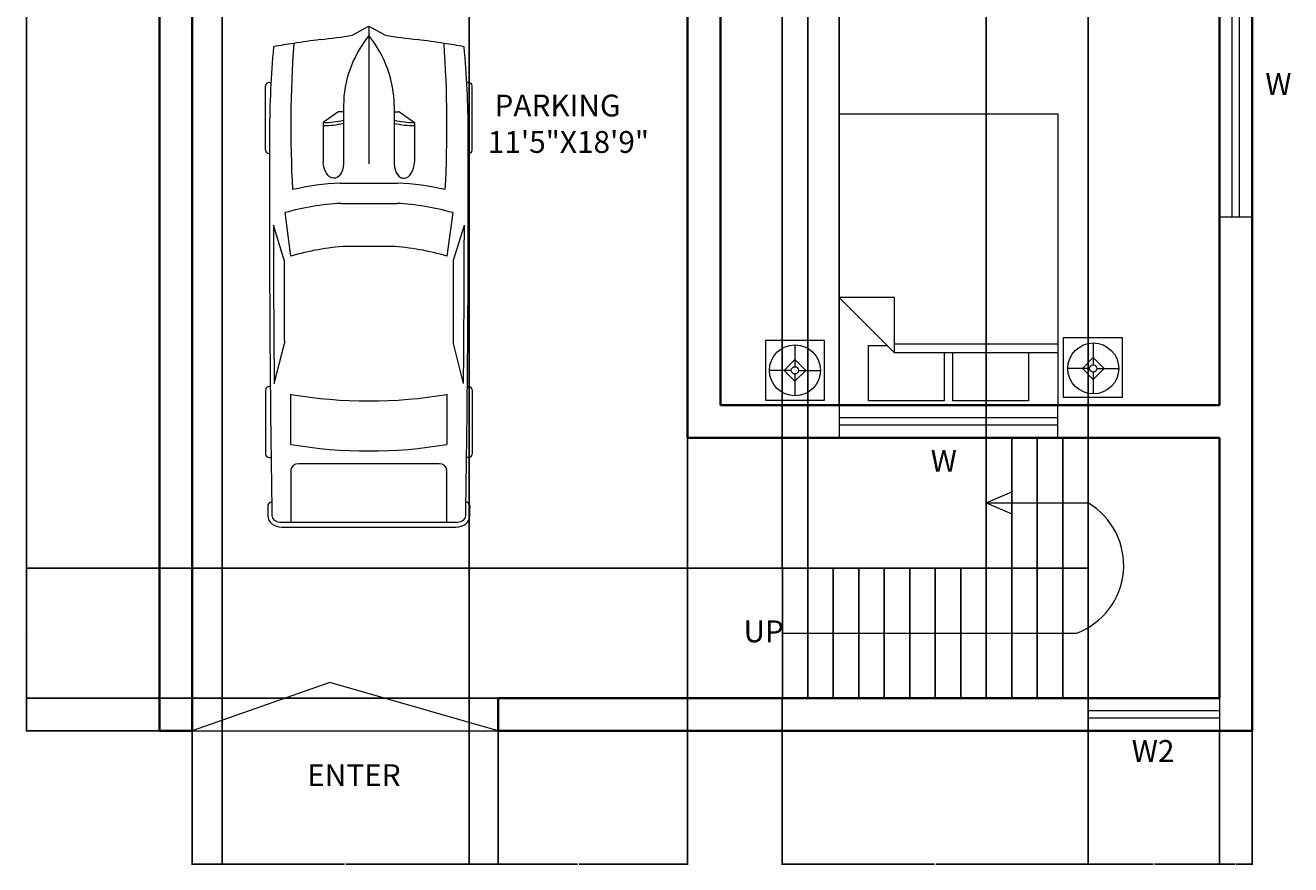
# Model space of a CAD drawing. Units: inches. Extents: x 2523 to 5630, y 2079 to 4208.
# Tile 1 of 3: x 2523 to 2870, y 2079 to 2309. Entities that reach past the tile are written whole.
import ezdxf

# ---------------------------------------------------------------- set-up
doc = ezdxf.new("R2010")
doc.units = ezdxf.units.IN
for name, color, linetype, lineweight in [('A-ANNO-DIMS', 2, 'Continuous', 18), ('A-ANNO-SYMB', 2, 'Continuous', 18), ('A-ANNO-TEXT', 7, 'Continuous', 18), ('A-AREA-IDEN', 7, 'Continuous', 25), ('A-EQPM-VEHC', 9, 'Continuous', 13), ('A-FLOR-STRS', 7, 'Continuous', 25), ('A-FURN', 8, 'Continuous', 18), ('A-GLAZ', 4, 'Continuous', 18), ('A-WALL', 7, 'Continuous', 35)]:
    doc.layers.add(name, color=color, linetype=linetype, lineweight=lineweight)
doc.styles.get("Standard").update_dxf_attribs({"font": 'arial.ttf'})
doc.dimstyles.get("Standard").update_dxf_attribs({"dimtxt": 0.18, "dimasz": 0.18, "dimexe": 0.18, "dimexo": 0.0625, "dimgap": 0.09, "dimtad": 0, "dimtih": 1, "dimtoh": 1, "dimdec": 4, "dimzin": 0, "dimdsep": 46, "dimtxsty": 'Standard', "dimcen": 0.09, "dimadec": 0, "dimazin": 0, "dimtfac": 1, "dimtdec": 4, "dimtofl": 0, "dimtmove": 0, "dimatfit": 3, "dimfxl": 1, "dimtolj": 1, "dimtzin": 0, "dimarcsym": 0})

# ---------------------------------------------------------------- blocks, each defined once
blk = doc.blocks.new('Bed - Queen')
for p, q in [((0, -80.00003), (0, 0)), ((0, 0), (59.99999, 0)), ((59.99999, 0), (59.99999, -80.00003)), ((7.99999, -1.2), (28.79998, -1.2)), ((7.99999, -14.4), (7.99999, -1.2)), ((28.79998, -1.2), (28.79998, -14.4)), ((31.19999, -1.2), (51.99999, -1.2)), ((31.19999, -14.4), (31.19999, -1.2)), ((51.99999, -1.2), (51.99999, -16.4)), ((0, -14.4), (44.8, -14.4)), ((44.8, -16.8), (0, -16.8)), ((59.99999, -29.6), (44.8, -14.4)), ((44.8, -14.4), (44.8, -29.6)), ((51.99999, -16.4), (46.79936, -16.4)), ((44.8, -29.6), (59.99999, -29.6)), ((59.99999, -80.00003), (0, -80.00003))]:
    blk.add_line(p, q)
blk = doc.blocks.new('Lamp - Table')
for p, q in [((0, 7), (0, 1)), ((-1, 0), (-7, 0)), ((0, 3), (-3, 0)), ((-3, 0), (0, -3)), ((3, 0), (0, 3)), ((0, -3), (3, 0)), ((1, 0), (7, 0)), ((0, -1), (0, -7))]:
    blk.add_line(p, q)
for radius in [7, 1]:
    blk.add_circle((0, 0), radius)
blk = doc.blocks.new('*U9')
for p, q in [((46.55, 38.89), (22.35, 38.89)), ((136.7, 38.89), (160.9, 38.89)), ((21.1, 37.41), (21.1, 36.83)), ((47.8, 37.39), (47.8, 37.41)), ((87.99, 31.87), (74.76, 35.92)), ((134.31, 35.6), (119.29, 31.78)), ((135.45, 37.07), (135.45, 37.41)), ((162.15, 37.41), (162.15, 36.77)), ((186.47, -33.5), (186.47, 33.5)), ((70.03, 31.54), (86.41, 29.35)), ((138.42, 29.35), (157.25, 29.35)), ((186.47, 29.35), (167.01, 29.35)), ((188.4, -32.76), (188.4, 32.76)), ((164.52, 26.39), (164.52, -26.39)), ((32.27, 11.63), (36.13, 17.17)), ((36.13, 17.17), (50.94, 17.17)), ((32.12, 9.51), (32.12, 11.15)), ((58.92, -10.77), (58.92, 10.77)), ((66.55, -10.53), (66.55, 10.53)), ((186.47, -10.53), (186.47, 10.53)), ((3.27, 6.13), (0.1, 0.41)), ((29.77, 9.51), (51.68, 9.51)), ((82.74, 8.5), (82.74, -8.5)), ((0, 0), (51.68, 0)), ((0.1, -0.41), (3.27, -6.13)), ((29.77, -9.51), (51.68, -9.51)), ((32.12, -9.51), (32.12, -11.15)), ((32.27, -11.63), (36.13, -17.17)), ((36.13, -17.17), (50.94, -17.17)), ((86.41, -29.35), (70.03, -31.54)), ((87.99, -31.87), (74.76, -35.92)), ((134.31, -35.6), (119.29, -31.78)), ((157.25, -29.35), (138.42, -29.35)), ((167.01, -29.35), (186.47, -29.35)), ((21.1, -37.41), (21.1, -36.83)), ((47.8, -37.39), (47.8, -37.41)), ((135.45, -37.07), (135.45, -37.41)), ((162.15, -37.41), (162.15, -36.77)), ((46.55, -38.89), (22.35, -38.89)), ((136.7, -38.89), (160.9, -38.89))]:
    blk.add_line(p, q)
for centre, major_axis, ratio, start_param, end_param in [((22.35, 37.41), (0, -1.48), 0.842304, 3.141593, 4.712389), ((46.55, 37.41), (0, 1.48), 0.842304, -1.570796, 0), ((136.7, 37.41), (0, -1.48), 0.842304, 3.141593, 4.712389), ((160.9, 37.41), (0, 1.48), 0.842304, -1.570796, 0), ((266.03, -27.52), (0, 313.31), 0.842304, 1.367076, 1.39176), ((41.19, -490.86), (0, 528.23), 0.842304, 0.00281, 0.075598), ((64.48, -10555.62), (0, 10593.03), 0.842304, -0.013397, 0.002797), ((64.48, -10555.62), (0, -10591.55), 0.842304, 3.133765, 3.140441), ((180.63, 35.84), (0, 2.22), 0.842304, -0.013017, 1.249894), ((64.48, -10556.36), (0, 10595.31), 0.842304, -0.013397, -0.013017), ((183.98, 33.5), (0, -2.96), 0.842304, 1.570796, 3.128196), ((183.98, 32.76), (0, -5.25), 0.842304, 1.570796, 3.128196), ((37.47, -593.96), (0, -623.33), 0.842304, 3.096046, 3.200911), ((134.4, 5.39), (0, -89.78), 0.842304, 4.449482, 4.652344), ((135.29, 5.39), (0, 81.77), 0.842304, 1.245306, 1.50788), ((149.6, 2.8), (0, -79.58), 0.842304, 4.372215, 4.640744), ((95.79, -3666.35), (0, -3698.24), 0.842304, 3.134049, 3.144098), ((17.08, 0), (0, 147.02), 0.842304, 4.511394, 4.913384), ((35.91, 0), (0, 147.02), 0.842304, 4.511394, 4.913384), ((167.01, 26.39), (0, 2.96), 0.842304, 0, 1.570796), ((259.18, -27.52), (0, -305.3), 0.842304, 4.528606, 4.561838), ((-204.49, 52.4), (0, -250.96), 0.842304, 1.385369, 1.434372), ((13.04, 17.01), (0, 27.42), 0.842304, 4.435146, 4.718221), ((14.2, 17.01), (0, 27.42), 0.842304, 4.435146, 4.718221), ((50.79, 13.34), (6.34, -0.36), 0.603834, -1.395552, 1.581315), ((32.75, 11.15), (0, 0.74), 0.842304, 0.879714, 1.570796), ((29.77, -46.66), (0, 56.17), 0.842304, 0, 0.590319), ((0.62, 0), (0, -0.74), 0.842304, 4.131459, 5.293319), ((29.77, 46.66), (0, 56.17), 0.842304, 2.551274, 3.141593), ((-204.49, -52.4), (0, 250.96), 0.842304, -1.434372, -1.385369), ((13.04, -17.01), (0, -27.42), 0.842304, 1.564964, 1.848039), ((14.2, -17.01), (0, -27.42), 0.842304, 1.564964, 1.848039), ((149.6, -2.8), (0, -79.58), 0.842304, -1.499151, -1.230623), ((32.75, -11.15), (0, -0.74), 0.842304, 4.712389, 5.403472), ((134.4, -5.39), (0, -89.78), 0.842304, -1.510751, -1.307889), ((135.29, -5.39), (0, -81.77), 0.842304, -1.50788, -1.245306), ((259.18, 27.52), (0, 305.3), 0.842304, 1.721348, 1.754579), ((266.03, 27.52), (0, 313.31), 0.842304, 1.749832, 1.774517), ((37.47, 593.96), (0, -623.33), 0.842304, -0.059319, 0.045547), ((167.01, -26.39), (0, -2.96), 0.842304, 4.712389, 6.283185), ((95.79, 3666.35), (0, -3698.24), 0.842304, -0.002505, 0.007544), ((183.98, -32.76), (0, -5.25), 0.842304, 0.013397, 1.570796), ((41.19, 490.86), (0, -528.23), 0.842304, -0.075598, -0.00281), ((22.35, -37.41), (0, 1.48), 0.842304, 1.570796, 3.141593), ((64.48, 10555.62), (0, 10593.03), 0.842304, 3.138796, 3.15499), ((46.55, -37.41), (0, -1.48), 0.842304, 0, 1.570796), ((64.48, 10555.62), (0, -10591.55), 0.842304, 0.001152, 0.007828), ((136.7, -37.41), (0, -1.48), 0.842304, -1.570796, 0), ((160.9, -37.41), (0, 1.48), 0.842304, 3.141593, 4.712389), ((180.63, -35.84), (0, -2.22), 0.842304, -1.249894, 0.013017), ((64.48, 10556.36), (0, 10595.31), 0.842304, 3.15461, 3.15499), ((183.98, -33.5), (0, 2.96), 0.842304, 3.15499, 4.712389)]:
    blk.add_ellipse(centre, major_axis=major_axis, ratio=ratio, start_param=start_param, end_param=end_param)
at = {"extrusion": (0, 0, -1)}
blk.add_ellipse((50.79, -13.34), major_axis=(6.34, 0.36), ratio=0.603834, start_param=-1.395552, end_param=1.581315, dxfattribs=at)
blk = doc.blocks.new('WIN-W-60IN')
for p, q in [((60, 5.5), (0, 5.5)), ((60, 3.5), (0, 3.5))]:
    blk.add_line(p, q)
blk.add_lwpolyline([(0, 0), (60, 0), (60, 9), (0, 9)], close=True)
blk = doc.blocks.new('TABLE-BEDSIDE')
blk.add_lwpolyline([(0, 0), (16.27, 0), (16.27, 16.36), (0, 16.36)], close=True)
blk = doc.blocks.new('*D33')
at = {"layer": 'A-ANNO-DIMS', "color": 0, "lineweight": -2, "transparency": 16777216}
for p, q in [((2559.63, 2775.33), (2522.96, 2775.33)), ((2523.14, 2775.15), (2523.14, 2445.52)), ((2523.14, 2115.51), (2523.14, 2445.15)), ((2559.63, 2115.33), (2522.96, 2115.33))]:
    blk.add_line(p, q, dxfattribs=at)
at = {"layer": 'A-ANNO-DIMS', "color": 0, "transparency": 16777216}
for points in [[(2523.11, 2775.15), (2523.17, 2775.15), (2523.14, 2775.33)], [(2523.11, 2115.51), (2523.17, 2115.51), (2523.14, 2115.33)]]:
    blk.add_solid(points, dxfattribs=at)
at = {"layer": 'Defpoints', "color": 0, "transparency": 16777216}
for p in [(2523.14, 2775.33), (2559.69, 2775.33), (2559.69, 2115.33)]:
    blk.add_point(p, dxfattribs=at)
at = {"layer": 'A-ANNO-DIMS', "color": 0, "transparency": 16777216, "insert": (2523.14, 2445.33), "char_height": 0.18, "attachment_point": 5}
blk.add_mtext('\\A1;660', dxfattribs=at)
blk = doc.blocks.new('*D34')
at = {"layer": 'A-ANNO-DIMS', "color": 0, "lineweight": -2, "transparency": 16777216}
for p, q in [((2568.69, 2115.27), (2568.69, 2078.6)), ((2652.69, 2115.27), (2652.69, 2078.6)), ((2568.87, 2078.78), (2610.47, 2078.78)), ((2652.51, 2078.78), (2610.91, 2078.78))]:
    blk.add_line(p, q, dxfattribs=at)
at = {"layer": 'A-ANNO-DIMS', "color": 0, "transparency": 16777216}
for points in [[(2568.87, 2078.81), (2568.87, 2078.75), (2568.69, 2078.78)], [(2652.51, 2078.81), (2652.51, 2078.75), (2652.69, 2078.78)]]:
    blk.add_solid(points, dxfattribs=at)
at = {"layer": 'Defpoints', "color": 0, "transparency": 16777216}
for p in [(2568.69, 2115.33), (2652.69, 2115.33), (2652.69, 2078.78)]:
    blk.add_point(p, dxfattribs=at)
at = {"layer": 'A-ANNO-DIMS', "color": 0, "transparency": 16777216, "insert": (2610.69, 2078.78), "char_height": 0.18, "attachment_point": 5}
blk.add_mtext('\\A1;84', dxfattribs=at)
blk = doc.blocks.new('*D35')
at = {"layer": 'A-ANNO-DIMS', "color": 0, "lineweight": -2, "transparency": 16777216}
for p, q in [((2814.69, 2115.27), (2814.69, 2078.6)), ((2850.69, 2115.27), (2850.69, 2078.6)), ((2814.87, 2078.78), (2832.47, 2078.78)), ((2850.51, 2078.78), (2832.91, 2078.78))]:
    blk.add_line(p, q, dxfattribs=at)
at = {"layer": 'A-ANNO-DIMS', "color": 0, "transparency": 16777216}
for points in [[(2814.87, 2078.81), (2814.87, 2078.75), (2814.69, 2078.78)], [(2850.51, 2078.81), (2850.51, 2078.75), (2850.69, 2078.78)]]:
    blk.add_solid(points, dxfattribs=at)
at = {"layer": 'Defpoints', "color": 0, "transparency": 16777216}
for p in [(2814.69, 2115.33), (2850.69, 2115.33), (2850.69, 2078.78)]:
    blk.add_point(p, dxfattribs=at)
at = {"layer": 'A-ANNO-DIMS', "color": 0, "transparency": 16777216, "insert": (2832.69, 2078.78), "char_height": 0.18, "attachment_point": 5}
blk.add_mtext('\\A1;36', dxfattribs=at)
blk = doc.blocks.new('*D36')
at = {"layer": 'A-ANNO-DIMS', "color": 0, "lineweight": -2, "transparency": 16777216}
for p, q in [((2704.69, 2353.27), (2704.69, 2078.6)), ((2644.69, 2348.77), (2644.69, 2078.6)), ((2644.87, 2078.78), (2674.47, 2078.78)), ((2704.51, 2078.78), (2674.91, 2078.78))]:
    blk.add_line(p, q, dxfattribs=at)
at = {"layer": 'A-ANNO-DIMS', "color": 0, "transparency": 16777216}
for points in [[(2644.87, 2078.81), (2644.87, 2078.75), (2644.69, 2078.78)], [(2704.51, 2078.81), (2704.51, 2078.75), (2704.69, 2078.78)]]:
    blk.add_solid(points, dxfattribs=at)
at = {"layer": 'Defpoints', "color": 0, "transparency": 16777216}
for p in [(2704.69, 2353.33), (2644.69, 2348.83), (2704.69, 2078.78)]:
    blk.add_point(p, dxfattribs=at)
at = {"layer": 'A-ANNO-DIMS', "color": 0, "transparency": 16777216, "insert": (2674.69, 2078.78), "char_height": 0.18, "attachment_point": 5}
blk.add_mtext('\\A1;60', dxfattribs=at)
blk = doc.blocks.new('*D37')
at = {"layer": 'A-ANNO-DIMS', "color": 0, "lineweight": -2, "transparency": 16777216}
for p, q in [((2850.69, 2115.27), (2850.69, 2078.6)), ((2859.69, 2115.27), (2859.69, 2078.6)), ((2850.87, 2078.78), (2855.04, 2078.78)), ((2859.51, 2078.78), (2855.34, 2078.78))]:
    blk.add_line(p, q, dxfattribs=at)
at = {"layer": 'A-ANNO-DIMS', "color": 0, "transparency": 16777216}
for points in [[(2850.87, 2078.81), (2850.87, 2078.75), (2850.69, 2078.78)], [(2859.51, 2078.81), (2859.51, 2078.75), (2859.69, 2078.78)]]:
    blk.add_solid(points, dxfattribs=at)
at = {"layer": 'Defpoints', "color": 0, "transparency": 16777216}
for p in [(2850.69, 2115.33), (2859.69, 2115.33), (2859.69, 2078.78)]:
    blk.add_point(p, dxfattribs=at)
at = {"layer": 'A-ANNO-DIMS', "color": 0, "transparency": 16777216, "insert": (2855.19, 2078.78), "char_height": 0.18, "attachment_point": 5}
blk.add_mtext('\\A1;9', dxfattribs=at)
blk = doc.blocks.new('*D38')
at = {"layer": 'A-ANNO-DIMS', "color": 0, "lineweight": -2, "transparency": 16777216}
for p, q in [((2730.69, 2124.27), (2730.69, 2078.6)), ((2814.69, 2124.27), (2814.69, 2078.6)), ((2730.87, 2078.78), (2772.47, 2078.78)), ((2814.51, 2078.78), (2772.91, 2078.78))]:
    blk.add_line(p, q, dxfattribs=at)
at = {"layer": 'A-ANNO-DIMS', "color": 0, "transparency": 16777216}
for points in [[(2730.87, 2078.81), (2730.87, 2078.75), (2730.69, 2078.78)], [(2814.51, 2078.81), (2814.51, 2078.75), (2814.69, 2078.78)]]:
    blk.add_solid(points, dxfattribs=at)
at = {"layer": 'Defpoints', "color": 0, "transparency": 16777216}
for p in [(2730.69, 2124.33), (2814.69, 2124.33), (2814.69, 2078.78)]:
    blk.add_point(p, dxfattribs=at)
at = {"layer": 'A-ANNO-DIMS', "color": 0, "transparency": 16777216, "insert": (2772.69, 2078.78), "char_height": 0.18, "attachment_point": 5}
blk.add_mtext('\\A1;84', dxfattribs=at)
blk = doc.blocks.new('*D39')
at = {"layer": 'A-ANNO-DIMS', "color": 0, "lineweight": -2, "transparency": 16777216}
for p, q in [((2730.63, 2160.08), (2522.96, 2160.08)), ((2523.14, 2159.9), (2523.14, 2142.39)), ((2523.14, 2124.51), (2523.14, 2142.03)), ((2730.63, 2124.33), (2522.96, 2124.33))]:
    blk.add_line(p, q, dxfattribs=at)
at = {"layer": 'A-ANNO-DIMS', "color": 0, "transparency": 16777216}
for points in [[(2523.11, 2159.9), (2523.17, 2159.9), (2523.14, 2160.08)], [(2523.11, 2124.51), (2523.17, 2124.51), (2523.14, 2124.33)]]:
    blk.add_solid(points, dxfattribs=at)
at = {"layer": 'Defpoints', "color": 0, "transparency": 16777216}
for p in [(2523.14, 2160.08), (2730.69, 2160.08), (2730.69, 2124.33)]:
    blk.add_point(p, dxfattribs=at)
at = {"layer": 'A-ANNO-DIMS', "color": 0, "transparency": 16777216, "insert": (2523.14, 2142.21), "char_height": 0.18, "attachment_point": 5}
blk.add_mtext('\\A1;35.75', dxfattribs=at)
blk = doc.blocks.new('*D40')
at = {"layer": 'A-ANNO-DIMS', "color": 0, "lineweight": -2, "transparency": 16777216}
for p, q in [((2786.69, 2195.9), (2786.69, 2812.06)), ((2786.87, 2811.88), (2800.47, 2811.88)), ((2814.51, 2811.88), (2800.91, 2811.88)), ((2814.69, 2195.9), (2814.69, 2812.06))]:
    blk.add_line(p, q, dxfattribs=at)
at = {"layer": 'A-ANNO-DIMS', "color": 0, "transparency": 16777216}
for points in [[(2786.87, 2811.91), (2786.87, 2811.85), (2786.69, 2811.88)], [(2814.51, 2811.91), (2814.51, 2811.85), (2814.69, 2811.88)]]:
    blk.add_solid(points, dxfattribs=at)
at = {"layer": 'Defpoints', "color": 0, "transparency": 16777216}
for p in [(2814.69, 2811.88), (2786.69, 2195.83), (2814.69, 2195.83)]:
    blk.add_point(p, dxfattribs=at)
at = {"layer": 'A-ANNO-DIMS', "color": 0, "transparency": 16777216, "insert": (2800.69, 2811.88), "char_height": 0.18, "attachment_point": 5}
blk.add_mtext('\\A1;28', dxfattribs=at)
blk = doc.blocks.new('*D41')
at = {"layer": 'A-ANNO-DIMS', "color": 0, "lineweight": -2, "transparency": 16777216}
for p, q in [((2730.69, 2160.15), (2730.69, 2812.06)), ((2730.87, 2811.88), (2734.04, 2811.88)), ((2737.51, 2811.88), (2734.34, 2811.88)), ((2737.69, 2160.15), (2737.69, 2812.06))]:
    blk.add_line(p, q, dxfattribs=at)
at = {"layer": 'A-ANNO-DIMS', "color": 0, "transparency": 16777216}
for points in [[(2730.87, 2811.91), (2730.87, 2811.85), (2730.69, 2811.88)], [(2737.51, 2811.91), (2737.51, 2811.85), (2737.69, 2811.88)]]:
    blk.add_solid(points, dxfattribs=at)
at = {"layer": 'Defpoints', "color": 0, "transparency": 16777216}
for p in [(2737.69, 2811.88), (2730.69, 2160.08), (2737.69, 2160.08)]:
    blk.add_point(p, dxfattribs=at)
at = {"layer": 'A-ANNO-DIMS', "color": 0, "transparency": 16777216, "insert": (2734.19, 2811.88), "char_height": 0.18, "attachment_point": 5}
blk.add_mtext('\\A1;7', dxfattribs=at)
blk = doc.blocks.new('*D47')
at = {"layer": 'A-ANNO-DIMS', "color": 0, "lineweight": -2, "transparency": 16777216}
for p, q in [((2568.69, 2348.77), (2568.69, 2078.6)), ((2576.87, 2348.77), (2576.87, 2078.6)), ((2568.87, 2078.78), (2572.39, 2078.78)), ((2576.69, 2078.78), (2573.17, 2078.78))]:
    blk.add_line(p, q, dxfattribs=at)
at = {"layer": 'A-ANNO-DIMS', "color": 0, "transparency": 16777216}
for points in [[(2568.87, 2078.81), (2568.87, 2078.75), (2568.69, 2078.78)], [(2576.69, 2078.81), (2576.69, 2078.75), (2576.87, 2078.78)]]:
    blk.add_solid(points, dxfattribs=at)
at = {"layer": 'Defpoints', "color": 0, "transparency": 16777216}
for p in [(2568.69, 2348.83), (2576.87, 2348.83), (2576.87, 2078.78)]:
    blk.add_point(p, dxfattribs=at)
at = {"layer": 'A-ANNO-DIMS', "color": 0, "transparency": 16777216, "insert": (2572.78, 2078.78), "char_height": 0.18, "attachment_point": 5}
blk.add_mtext('\\A1;8.174', dxfattribs=at)
blk = doc.blocks.new('*D49')
at = {"layer": 'A-ANNO-DIMS', "color": 0, "lineweight": -2, "transparency": 16777216}
for p, q in [((2713.69, 2204.9), (2713.69, 2812.06)), ((2713.87, 2811.88), (2729.54, 2811.88)), ((2746.14, 2811.88), (2730.47, 2811.88)), ((2746.32, 2204.9), (2746.32, 2812.06))]:
    blk.add_line(p, q, dxfattribs=at)
at = {"layer": 'A-ANNO-DIMS', "color": 0, "transparency": 16777216}
for points in [[(2713.87, 2811.91), (2713.87, 2811.85), (2713.69, 2811.88)], [(2746.14, 2811.91), (2746.14, 2811.85), (2746.32, 2811.88)]]:
    blk.add_solid(points, dxfattribs=at)
at = {"layer": 'Defpoints', "color": 0, "transparency": 16777216}
for p in [(2746.32, 2811.88), (2713.69, 2204.83), (2746.32, 2204.83)]:
    blk.add_point(p, dxfattribs=at)
at = {"layer": 'A-ANNO-DIMS', "color": 0, "transparency": 16777216, "insert": (2730.01, 2811.88), "char_height": 0.18, "attachment_point": 5}
blk.add_mtext('\\A1;32.625', dxfattribs=at)

msp = doc.modelspace()

# ---------------------------------------------------------------- linework, layer by layer
at = {"layer": 'A-ANNO-SYMB'}
for p, q in [((2786.693, 2177.959), (2793.693, 2180.9837)), ((2786.693, 2177.959), (2814.693, 2177.959)), ((2786.693, 2177.959), (2793.693, 2174.9344)), ((2730.693, 2142.209), (2811.5066, 2142.209)), ((2606.4661, 2128.6189), (2568.693, 2115.334)), ((2652.693, 2115.334), (2606.4661, 2128.6189)), ((2568.693, 2115.334), (2652.693, 2115.334))]:
    msp.add_line(p, q, dxfattribs=at)
msp.add_arc((2804.4997, 2160.8506), 19.9149, 290.600004, 59.213206, dxfattribs=at)
at = {"layer": 'A-FLOR-STRS'}
for p, q in [((2786.693, 2160.084), (2786.693, 2195.834)), ((2793.693, 2160.084), (2793.693, 2195.834)), ((2800.693, 2160.084), (2800.693, 2195.834)), ((2807.693, 2160.084), (2807.693, 2195.834)), ((2814.693, 2160.084), (2814.693, 2195.834)), ((2814.693, 2160.084), (2730.693, 2160.084)), ((2730.693, 2124.334), (2730.693, 2160.084)), ((2737.693, 2124.334), (2737.693, 2160.084)), ((2744.693, 2124.334), (2744.693, 2160.084)), ((2751.693, 2124.334), (2751.693, 2160.084)), ((2758.693, 2124.334), (2758.693, 2160.084)), ((2765.693, 2124.334), (2765.693, 2160.084)), ((2772.693, 2124.334), (2772.693, 2160.084)), ((2779.693, 2124.334), (2779.693, 2160.084)), ((2786.693, 2124.334), (2786.693, 2160.084)), ((2793.693, 2124.334), (2793.693, 2160.084)), ((2800.693, 2124.334), (2800.693, 2160.084)), ((2807.693, 2124.334), (2807.693, 2160.084)), ((2814.693, 2124.334), (2814.693, 2160.084))]:
    msp.add_line(p, q, dxfattribs=at)
at = {"layer": 'A-GLAZ'}
for p, q in [((2850.693, 2120.834), (2814.693, 2120.834)), ((2850.693, 2118.834), (2814.693, 2118.834))]:
    msp.add_line(p, q, dxfattribs=at)
msp.add_lwpolyline([(2814.693, 2115.334), (2814.693, 2124.334), (2850.693, 2124.334), (2850.693, 2115.334)], close=True, dxfattribs=at)
at = {"layer": 'A-WALL'}
for p, q in [((2704.693, 2195.834), (2704.693, 2357.834)), ((2713.693, 2204.834), (2713.693, 2357.834)), ((2568.693, 2348.834), (2568.693, 2124.334)), ((2850.693, 2204.834), (2850.693, 2348.834)), ((2850.693, 2204.834), (2713.693, 2204.834)), ((2850.693, 2195.834), (2704.693, 2195.834)), ((2850.693, 2124.334), (2850.693, 2195.834)), ((2568.693, 2124.334), (2568.693, 2115.334)), ((2652.693, 2124.334), (2850.693, 2124.334)), ((2652.693, 2124.334), (2652.693, 2115.334))]:
    msp.add_line(p, q, dxfattribs=at)
msp.add_lwpolyline([(2652.693, 2115.334), (2859.693, 2115.334), (2859.693, 2775.334), (2559.693, 2775.334), (2559.693, 2115.334), (2568.693, 2115.334)], dxfattribs=at)

# ---------------------------------------------------------------- block references
at = {"layer": 'A-EQPM-VEHC', "xscale": 0.7298593814119692, "yscale": 0.7298593814119692, "zscale": 0.7298593814119692, "rotation": 270}
msp.add_blockref('*U9', (2617.1644, 2308.8317), dxfattribs=at)
at = {"layer": 'A-FURN', "rotation": 180}
msp.add_blockref('Bed - Queen', (2806.3179, 2204.834), dxfattribs=at)
at = {"layer": 'A-FURN'}
for name, p in [('TABLE-BEDSIDE', (2726.0257, 2206.2134)), ('Lamp - Table', (2734.1605, 2214.393)), ('TABLE-BEDSIDE', (2807.81, 2206.981)), ('Lamp - Table', (2816.0668, 2214.9045))]:
    msp.add_blockref(name, p, dxfattribs=at)
at = {"layer": 'A-GLAZ', "rotation": 270.0000000000015}
msp.add_blockref('WIN-W-60IN', (2850.693, 2316.5883), dxfattribs=at)
at = {"layer": 'A-GLAZ'}
msp.add_blockref('WIN-W-60IN', (2746.3179, 2195.834), dxfattribs=at)

# ---------------------------------------------------------------- texts
at = {"layer": 'A-ANNO-TEXT', "char_height": 6, "attachment_point": 1}
for s, insert in [('W', (2863.304, 2296.0291)), ('W', (2771.4285, 2192.547)), ('UP', (2720.0329, 2145.7002)), ('W2', (2826.6189, 2112.834)), ('ENTER', (2600.2329, 2106.1993))]:
    msp.add_mtext_dynamic_manual_height_columns(s, width=48.58232, gutter_width=12.5, heights=[0], dxfattribs=dict(at, insert=insert))
at = {"layer": 'A-AREA-IDEN', "insert": (2649.8271, 2290.1268), "char_height": 6, "attachment_point": 1}
msp.add_mtext_dynamic_manual_height_columns(' PARKING\\P11\'5"X18\'9"', width=48.58232, gutter_width=12.5, heights=[0], dxfattribs=at)

# ---------------------------------------------------------------- dimensions: what is measured, and where the dimension line sits
at = {"layer": 'A-ANNO-DIMS'}
for base, p1, p2, override, picture, middle in [((2746.3179, 2811.884), (2713.693, 2204.834), (2746.3179, 2204.834), {"dimdec": 3, "dimlfac": 1, "dimrnd": 0, "dimzin": 0, "dimdsep": 46, "dimlunit": 2}, '*D49', (2730.0055, 2811.884)), ((2737.693, 2811.884), (2730.693, 2160.084), (2737.693, 2160.084), {"dimdec": 0, "dimlfac": 1, "dimrnd": 0, "dimzin": 0, "dimdsep": 46, "dimlunit": 2}, '*D41', (2734.193, 2811.884)), ((2814.693, 2811.884), (2786.693, 2195.834), (2814.693, 2195.834), {"dimdec": 0, "dimlfac": 1, "dimrnd": 0, "dimzin": 0, "dimdsep": 46, "dimlunit": 2}, '*D40', (2800.693, 2811.884)), ((2704.693, 2078.784), (2644.693, 2348.834), (2704.693, 2353.334), {"dimdec": 0, "dimlfac": 1, "dimrnd": 0, "dimzin": 0, "dimdsep": 46, "dimlunit": 2}, '*D36', (2674.693, 2078.784)), ((2576.867, 2078.784), (2568.693, 2348.834), (2576.867, 2348.834), {"dimdec": 3, "dimlfac": 1, "dimrnd": 0, "dimzin": 0, "dimdsep": 46, "dimlunit": 2}, '*D47', (2572.78, 2078.784)), ((2814.693, 2078.784), (2730.693, 2124.334), (2814.693, 2124.334), {"dimdec": 0, "dimlfac": 1, "dimrnd": 0, "dimzin": 0, "dimdsep": 46, "dimlunit": 2}, '*D38', (2772.693, 2078.784)), ((2652.693, 2078.784), (2568.693, 2115.334), (2652.693, 2115.334), {"dimdec": 0, "dimlfac": 1, "dimrnd": 0, "dimzin": 0, "dimdsep": 46, "dimlunit": 2}, '*D34', (2610.693, 2078.784)), ((2850.693, 2078.784), (2814.693, 2115.334), (2850.693, 2115.334), {"dimdec": 0, "dimlfac": 1, "dimrnd": 0, "dimzin": 0, "dimdsep": 46, "dimlunit": 2}, '*D35', (2832.693, 2078.784)), ((2859.693, 2078.784), (2850.693, 2115.334), (2859.693, 2115.334), {"dimdec": 0, "dimlfac": 1, "dimrnd": 0, "dimzin": 0, "dimdsep": 46, "dimlunit": 2}, '*D37', (2855.193, 2078.784))]:
    dim = msp.add_linear_dim(base=base, p1=p1, p2=p2, dimstyle='Standard', override=override, dxfattribs=at)
    dim.commit()
    dim.dimension.update_dxf_attribs({"geometry": picture, "text_midpoint": middle})
for base, p1, p2, override, picture, middle in [((2523.143, 2775.334), (2559.693, 2115.334), (2559.693, 2775.334), {"dimdec": 0, "dimlfac": 1, "dimrnd": 0, "dimzin": 0, "dimdsep": 46, "dimlunit": 2}, '*D33', (2523.143, 2445.334)), ((2523.143, 2160.084), (2730.693, 2124.334), (2730.693, 2160.084), {"dimdec": 2, "dimlfac": 1, "dimrnd": 0, "dimzin": 0, "dimdsep": 46, "dimlunit": 2}, '*D39', (2523.143, 2142.209))]:
    dim = msp.add_linear_dim(base=base, p1=p1, p2=p2, angle=90, dimstyle='Standard', override=override, dxfattribs=at)
    dim.commit()
    dim.dimension.update_dxf_attribs({"geometry": picture, "text_midpoint": middle})

doc.saveas('drawing.dxf')
